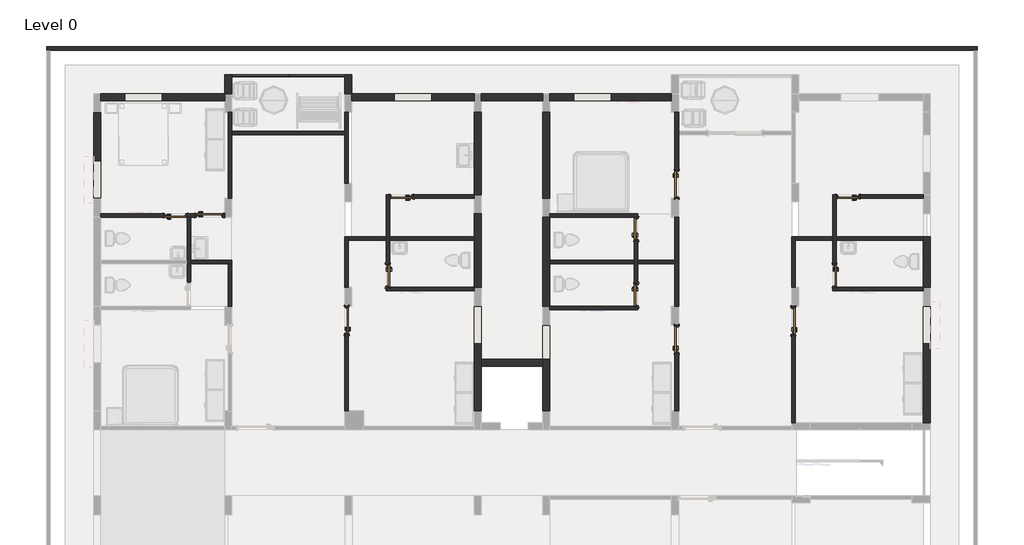
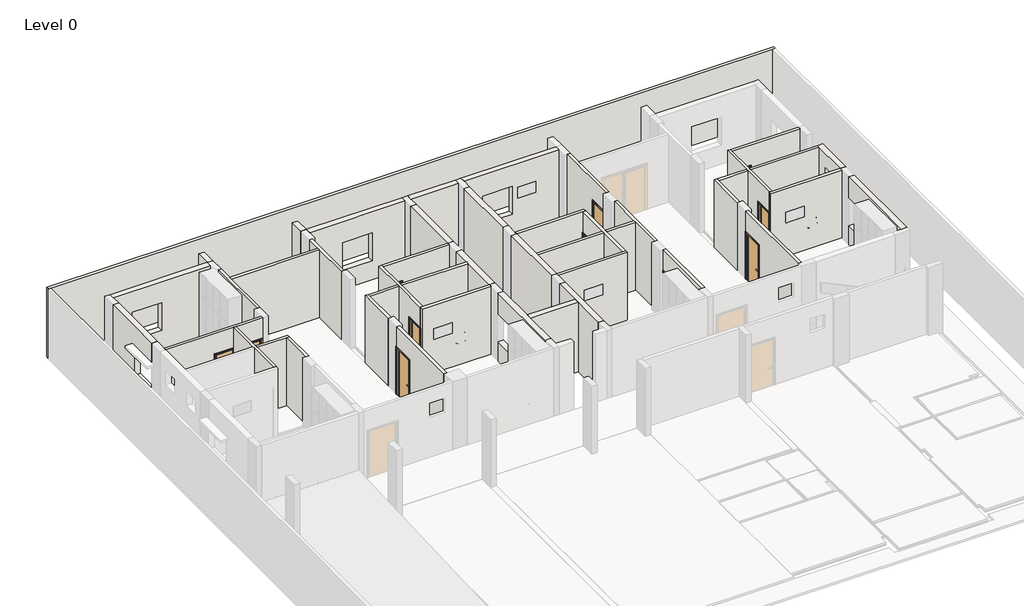
# One storey, part 2 of 6: 46 walls, 12 doors, 5 members, 2 plates.
"""IFC4 building model written with IfcOpenShell, lengths in millimetres."""

from ifc_helpers import new_model, si_unit, frame, origin, origin_with_axes, place, context, project, spatial, polyline, outline, extrude, faceted_brep, transform, mapped, element, save
from components import door_d225582b, door_4bb05ab8, doors_intsgl_3_11801b65, doors_intsgl_3_f3216364, rectangular_mullion_30mm_square_b78902bc, rectangular_mullion_30mm_square_5c6859bd, rectangular_mullion_30mm_square_457ab78e, rectangular_mullion_30mm_square_508dbaa4, system_panel_glazed_442d96c1, system_panel_glazed_6149afab

model = new_model("IFC4")

# Units and contexts
model_context = context("Model", 3, world=origin())
ifc_project = project(units=[si_unit("LENGTHUNIT", "METRE", prefix="MILLI")], contexts=[model_context])

# Site, building, storey
site = spatial("IfcSite", under=ifc_project)
building = spatial("IfcBuilding", under=site)
storey = spatial("IfcBuildingStorey", under=building, Name="Level 0", Elevation=0.0)

# Doors
placement = place(None, origin())
door_shape = door_d225582b(model_context)
element("IfcDoor", 1, ObjectType="Doors_IntSgl : 2'6\"", at=placement, inside=storey, context=model_context, shape_type="MappedRepresentation", body=[
    mapped(door_shape, transform((-10829.9825268, 6419.6522446, 0.0), x_axis=(1.0, 0.0, 0.0), y_axis=(0.0, 1.0, 0.0), z_axis=(0.0, 0.0, 1.0))),
])
element("IfcDoor", 2, ObjectType="Doors_IntSgl : 2'6\"", at=placement, inside=storey, context=model_context, shape_type="MappedRepresentation", body=[
    mapped(door_shape, transform((4085.7098461, 3836.3482139, 0.0), x_axis=(0.0, -1.0, 0.0), y_axis=(1.0, 0.0, 0.0), z_axis=(0.0, 0.0, 1.0))),
])
door_2_shape = door_4bb05ab8(model_context)
element("IfcDoor", 3, ObjectType="Doors_IntSgl : 2'6\"", at=placement, inside=storey, context=model_context, shape_type="MappedRepresentation", body=[
    mapped(door_2_shape, transform((-3954.0467595, 4470.172794, 0.0), x_axis=(-0.0005222285163052799, -0.9999998636386792, 0.0), y_axis=(0.9999998636386792, -0.0005222285163052799, 0.0), z_axis=(0.0, 0.0, 1.0))),
])
element("IfcDoor", 4, ObjectType="Doors_IntSgl : 2'6\"", at=placement, inside=storey, context=model_context, shape_type="MappedRepresentation", body=[
    mapped(door_2_shape, transform((-3514.5601716, 7029.4508507, 0.0), x_axis=(-0.9999998636386791, 0.000522228516302431, 0.0), y_axis=(-0.000522228516302431, -0.9999998636386791, 0.0), z_axis=(0.0, 0.0, 1.0))),
])
element("IfcDoor", 5, ObjectType="Doors_IntSgl : 2'6\"", at=placement, inside=storey, context=model_context, shape_type="MappedRepresentation", body=[
    mapped(door_2_shape, transform((4085.7098461, 5982.6482139, 0.0), x_axis=(0.0, 1.0, 0.0), y_axis=(-1.0, 0.0, 0.0), z_axis=(0.0, 0.0, 1.0))),
])
element("IfcDoor", 6, ObjectType="Doors_IntSgl : 2'6\"", at=placement, inside=storey, context=model_context, shape_type="MappedRepresentation", body=[
    mapped(door_2_shape, transform((10505.5598461, 4471.3482139, 0.0), x_axis=(0.0, -1.0, 0.0), y_axis=(1.0, 0.0, 0.0), z_axis=(0.0, 0.0, 1.0))),
])
element("IfcDoor", 7, ObjectType="Doors_IntSgl : 2'6\"", at=placement, inside=storey, context=model_context, shape_type="MappedRepresentation", body=[
    mapped(door_2_shape, transform((10943.7098461, 7030.3982139, 0.0), x_axis=(-1.0, 0.0, 0.0), y_axis=(0.0, -1.0, 0.0), z_axis=(0.0, 0.0, 1.0))),
])
doors_intsgl_3_shape = doors_intsgl_3_11801b65(model_context)
element("IfcDoor", 8, ObjectType="Doors_IntSgl : 3'", at=placement, inside=storey, context=model_context, shape_type="MappedRepresentation", body=[
    mapped(doors_intsgl_3_shape, transform((-9731.8901539, 6419.6522446, 0.0), x_axis=(1.0, 0.0, 0.0), y_axis=(0.0, 1.0, 0.0), z_axis=(0.0, 0.0, 1.0))),
])
element("IfcDoor", 9, ObjectType="Doors_IntSgl : 3'", at=placement, inside=storey, context=model_context, shape_type="MappedRepresentation", body=[
    mapped(doors_intsgl_3_shape, transform((5400.1598461, 2401.2482139, 0.0), x_axis=(0.0, 1.0, 0.0), y_axis=(-1.0, 0.0, 0.0), z_axis=(0.0, 0.0, 1.0))),
])
doors_intsgl_3_2_shape = doors_intsgl_3_f3216364(model_context)
element("IfcDoor", 10, ObjectType="Doors_IntSgl : 3'", at=placement, inside=storey, context=model_context, shape_type="MappedRepresentation", body=[
    mapped(doors_intsgl_3_2_shape, transform((-5287.3677108, 3023.5482139, 0.0), x_axis=(0.0, 1.0, 0.0), y_axis=(-1.0, 0.0, 0.0), z_axis=(0.0, 0.0, 1.0))),
])
element("IfcDoor", 11, ObjectType="Doors_IntSgl : 3'", at=placement, inside=storey, context=model_context, shape_type="MappedRepresentation", body=[
    mapped(doors_intsgl_3_2_shape, transform((5400.1598461, 7429.3022446, 0.0), x_axis=(0.0, -1.0, 0.0), y_axis=(1.0, 0.0, 0.0), z_axis=(0.0, 0.0, 1.0))),
])
element("IfcDoor", 12, ObjectType="Doors_IntSgl : 3'", at=placement, inside=storey, context=model_context, shape_type="MappedRepresentation", body=[
    mapped(doors_intsgl_3_2_shape, transform((9172.0598461, 2998.1482139, 0.0), x_axis=(0.0, 1.0, 0.0), y_axis=(-1.0, 0.0, 0.0), z_axis=(0.0, 0.0, 1.0))),
])

# Members
rectangular_mullion_30mm_square_shape = rectangular_mullion_30mm_square_b78902bc(model_context)
element("IfcMember", 13, ObjectType="Rectangular Mullion : 30mm_Square", at=placement, inside=storey, context=model_context, shape_type="MappedRepresentation", body=[
    mapped(rectangular_mullion_30mm_square_shape, transform((-7186.0406197, 10921.8022446, 1219.2), x_axis=(0.0, 0.0, 1.0), y_axis=(0.0, -1.0, 0.0), z_axis=(1.0, 0.0, 0.0))),
])
rectangular_mullion_30mm_square_2_shape = rectangular_mullion_30mm_square_5c6859bd(model_context)
element("IfcMember", 14, ObjectType="Rectangular Mullion : 30mm_Square", at=placement, inside=storey, context=model_context, shape_type="MappedRepresentation", body=[
    mapped(rectangular_mullion_30mm_square_2_shape, transform((-5374.0534022, 10921.8022446, 1219.2), x_axis=(0.0, 0.0, 1.0), y_axis=(0.0, -1.0, 0.0), z_axis=(1.0, 0.0, 0.0))),
])
rectangular_mullion_30mm_square_3_shape = rectangular_mullion_30mm_square_457ab78e(model_context)
element("IfcMember", 15, ObjectType="Rectangular Mullion : 30mm_Square", at=placement, inside=storey, context=model_context, shape_type="MappedRepresentation", body=[
    mapped(rectangular_mullion_30mm_square_3_shape, transform((-7171.0406197, 10921.8022446, 152.0481452), x_axis=(1.0, 0.0, 0.0), y_axis=(0.0, -1.0, 0.0), z_axis=(0.0, 0.0, -1.0))),
])
rectangular_mullion_30mm_square_4_shape = rectangular_mullion_30mm_square_508dbaa4(model_context)
element("IfcMember", 16, ObjectType="Rectangular Mullion : 30mm_Square", at=placement, inside=storey, context=model_context, shape_type="MappedRepresentation", body=[
    mapped(rectangular_mullion_30mm_square_4_shape, transform((-9001.04062, 10921.8022446, 1219.2), x_axis=(-1.0, 0.0, 0.0), y_axis=(0.0, -1.0, 0.0), z_axis=(0.0, 0.0, 1.0))),
])
element("IfcMember", 17, ObjectType="Rectangular Mullion : 30mm_Square", at=placement, inside=storey, context=model_context, shape_type="MappedRepresentation", body=[
    mapped(rectangular_mullion_30mm_square_4_shape, transform((-5344.0534022, 10921.8022446, 152.0481452), x_axis=(1.0, 0.0, 0.0), y_axis=(0.0, -1.0, 0.0), z_axis=(0.0, 0.0, -1.0))),
])

# Plates
system_panel_glazed_shape = system_panel_glazed_442d96c1(model_context)
element("IfcPlate", 18, ObjectType="System Panel : Glazed", at=placement, inside=storey, context=model_context, shape_type="MappedRepresentation", body=[
    mapped(system_panel_glazed_shape, transform((-8086.0406199, 10921.8022446, 152.0481452), x_axis=(1.0, 0.0, 0.0), y_axis=(0.0, 1.0, 0.0), z_axis=(0.0, 0.0, 1.0))),
])
system_panel_glazed_2_shape = system_panel_glazed_6149afab(model_context)
element("IfcPlate", 19, ObjectType="System Panel : Glazed", at=placement, inside=storey, context=model_context, shape_type="MappedRepresentation", body=[
    mapped(system_panel_glazed_2_shape, transform((-6257.547011, 10921.8022446, 152.0481452), x_axis=(1.0, 0.0, 0.0), y_axis=(0.0, 1.0, 0.0), z_axis=(0.0, 0.0, 1.0))),
])

# Walls
element("IfcWall", 20, ObjectType="2\"", at=placement, inside=storey, context=model_context, shape_type="SweptSolid", body=[
    extrude(outline(polyline([(-9001.04062, 10972.6022446), (-5344.0534022, 10972.6022446), (-5344.0534022, 10921.8022446), (-9001.04062, 10921.8022446), (-9001.04062, 10972.6022446)])), origin_with_axes(), (0.0, 0.0, 1.0), 152.0481452),
])
element("IfcWall", 21, ObjectType="9\"", at=placement, inside=storey, context=model_context, shape_type="SweptSolid", body=[
    extrude(outline(polyline([(0.0, -9230.2401539), (3048.0, -9230.2401539), (3048.0, -13249.7901539), (0.0, -13249.7901539), (0.0, -9230.2401539)]), holes=[polyline([(2133.6, -11248.7188871), (914.4, -11248.7188871), (914.4, -12467.9188871), (2133.6, -12467.9188871), (2133.6, -11248.7188871)])]), frame((0.0, 10133.2562752, 0.0), z_axis=(0.0, 1.0, 0.0), x_axis=(0.0, 0.0, 1.0)), (0.0, 0.0, 1.0), 228.6),
])
element("IfcWall", 22, ObjectType="9\"", at=placement, inside=storey, context=model_context, shape_type="SweptSolid", body=[
    extrude(outline(polyline([(0.0, -1153.0401539), (3048.0, -1153.0401539), (3048.0, -5115.4534022), (0.0, -5115.4534022), (0.0, -1153.0401539)]), holes=[polyline([(2133.6, -3743.8401538), (2133.6, -2524.6401538), (914.4, -2524.6401538), (914.4, -3743.8401538), (2133.6, -3743.8401538)])]), frame((0.0, 10134.4022446, 0.0), z_axis=(0.0, 1.0, 0.0), x_axis=(0.0, 0.0, 1.0)), (0.0, 0.0, 1.0), 228.6),
])
element("IfcWall", 23, ObjectType="9\"", at=placement, inside=storey, context=model_context, shape_type="SweptSolid", body=[
    extrude(outline(polyline([(1056.7598461, 10134.4022446), (-924.4401539, 10134.4022446), (-924.4401539, 10363.0022446), (1056.7598461, 10363.0022446), (1056.7598461, 10134.4022446)])), origin_with_axes(), (0.0, 0.0, 1.0), 3048.0),
])
element("IfcWall", 24, ObjectType="9\"", at=placement, inside=storey, context=model_context, shape_type="SweptSolid", body=[
    extrude(outline(polyline([(0.0, 1285.3598461), (0.0, 5228.7098461), (3048.0, 5228.7098461), (3048.0, 1285.3598461), (0.0, 1285.3598461)]), holes=[polyline([(2133.6, 3286.4311129), (914.4, 3286.4311129), (914.4, 2067.2311129), (2133.6, 2067.2311129), (2133.6, 3286.4311129)])]), frame((0.0, 10134.4022446, 0.0), z_axis=(0.0, 1.0, 0.0), x_axis=(0.0, 0.0, 1.0)), (0.0, 0.0, 1.0), 228.6),
])
element("IfcWall", 25, ObjectType="9\"", at=placement, inside=storey, context=model_context, shape_type="SweptSolid", body=[
    extrude(outline(polyline([(4090.3482139, 0.0), (4090.3482139, 3048.0), (5728.6482139, 3048.0), (5728.6482139, 0.0), (4090.3482139, 0.0)]), holes=[polyline([(5157.1482139, 2438.4), (4547.5482139, 2438.4), (4547.5482139, 1828.8), (5157.1482139, 1828.8), (5157.1482139, 2438.4)])]), frame((13382.1098465, 0.0, 0.0), z_axis=(1.0, 0.0, 0.0), x_axis=(0.0, 1.0, 0.0)), (0.0, 0.0, 1.0), 228.6),
])
element("IfcWall", 26, ObjectType="9\"", at=placement, inside=storey, context=model_context, shape_type="SweptSolid", body=[
    extrude(outline(polyline([(-3771.9, 0.0), (0.0, 0.0), (0.0, -3048.0), (-3771.9, -3048.0), (-3771.9, -2133.6), (-2552.7, -2133.6), (-2552.7, -914.4), (-3771.9, -914.4), (-3771.9, 0.0)])), frame((13382.1098461, -291.1517861, 0.0), z_axis=(1.0, -9.266855296587119e-11, 0.0), x_axis=(-9.266855296587119e-11, -1.0, 0.0)), (0.0, 0.0, 1.0), 228.6),
])
element("IfcWall", 27, ObjectType="9\"", at=placement, inside=storey, context=model_context, shape_type="SweptSolid", body=[
    extrude(outline(polyline([(9752.2562752, 0.0), (6972.1022446, 0.0), (6972.1022446, 914.4), (8190.1562752, 914.4), (8190.1562752, 2133.6), (6972.1022446, 2133.6), (6972.1022446, 3048.0), (9752.2562752, 3048.0), (9752.2562752, 0.0)])), frame((-13478.3901539, 0.0, 0.0), z_axis=(1.0, 0.0, 0.0), x_axis=(0.0, 1.0, 0.0)), (0.0, 0.0, 1.0), 228.6),
])
element("IfcWall", 28, ObjectType="9\"", at=placement, inside=storey, context=model_context, shape_type="SweptSolid", body=[
    extrude(outline(polyline([(-924.4401539, 7087.5482139), (-1153.0401539, 7087.5482139), (-1153.0401539, 9753.4022446), (-924.4401539, 9753.4022446), (-924.4401539, 7087.5482139)])), origin_with_axes(), (0.0, 0.0, 1.0), 3048.0),
])
element("IfcWall", 29, ObjectType="9\"", at=placement, inside=storey, context=model_context, shape_type="SweptSolid", body=[
    extrude(outline(polyline([(1056.7598461, 6972.1022446), (1056.7598461, 9753.4022446), (1285.3598461, 9753.4022446), (1285.3598461, 6972.1022446), (1056.7598461, 6972.1022446)])), origin_with_axes(), (0.0, 0.0, 1.0), 3048.0),
])
element("IfcWall", 30, ObjectType="9\"", at=placement, inside=storey, context=model_context, shape_type="SweptSolid", body=[
    extrude(outline(polyline([(1056.7598461, 3481.8941832), (1056.7598461, 6362.5022446), (1285.3598461, 6362.5022446), (1285.3598461, 3481.8941832), (1056.7598461, 3481.8941832)])), origin_with_axes(), (0.0, 0.0, 1.0), 3048.0),
])
element("IfcWall", 31, ObjectType="9\"", at=placement, inside=storey, context=model_context, shape_type="SweptSolid", body=[
    extrude(outline(polyline([(-1153.0401539, 4089.2022446), (-1153.0401539, 6477.9482139), (-924.4401539, 6477.9482139), (-924.4401539, 4089.2022446), (-1153.0401539, 4089.2022446)])), origin_with_axes(), (0.0, 0.0, 1.0), 3048.0),
])
element("IfcWall", 32, ObjectType="9\"", at=placement, inside=storey, context=model_context, shape_type="Brep", body=[
    faceted_brep([(-924.4401539, 89.8482139, 0.0), (-924.4401539, 1537.6482139, 0.0), (-924.4401539, 1766.2482139, 0.0), (-924.4401539, 3479.6022446, 0.0), (-924.4401539, 3479.6022446, 914.4), (-924.4401539, 2260.4022446, 914.4), (-924.4401539, 2260.4022446, 2133.6), (-924.4401539, 3479.6022446, 2133.6), (-924.4401539, 3479.6022446, 3048.0), (-924.4401539, 1766.2482139, 3048.0), (-924.4401539, 1537.6482139, 3048.0), (-924.4401539, 89.8482139, 3048.0), (-1153.0401539, 3479.6022446, 0.0), (-1153.0401539, 89.8482139, 0.0), (-1153.0401539, 89.8482139, 3048.0), (-1153.0401539, 3479.6022446, 3048.0), (-1153.0401539, 3479.6022446, 2133.6), (-1153.0401539, 2260.4022446, 2133.6), (-1153.0401539, 2260.4022446, 914.4), (-1153.0401539, 3479.6022446, 914.4)], [[[0, 1, 2, 3, 4, 5, 6, 7, 8, 9, 10, 11]], [[12, 13, 14, 15, 16, 17, 18, 19]], [[3, 2, 1, 0, 13, 12]], [[3, 12, 19, 4]], [[15, 8, 7, 16]], [[11, 10, 9, 8, 15, 14]], [[0, 11, 14, 13]], [[18, 5, 4, 19]], [[5, 18, 17, 6]], [[6, 17, 16, 7]]]),
])
element("IfcWall", 33, ObjectType="9\"", at=placement, inside=storey, context=model_context, shape_type="Brep", body=[
    faceted_brep([(1056.7598461, 2872.2941832, 0.0), (1056.7598461, 1766.2482139, 0.0), (1056.7598461, 1537.6482139, 0.0), (1056.7598461, 89.8482139, 0.0), (1056.7598461, 89.8482139, 3048.0), (1056.7598461, 1537.6482139, 3048.0), (1056.7598461, 1766.2482139, 3048.0), (1056.7598461, 2872.2941832, 3048.0), (1056.7598461, 2872.2941832, 2133.6), (1056.7598461, 1766.2482138, 2133.6), (1056.7598461, 1766.2482138, 914.4), (1056.7598461, 2872.2941832, 914.4), (1285.3598461, 89.8482139, 0.0), (1285.3598461, 2872.2941832, 0.0), (1285.3598461, 2872.2941832, 914.4), (1285.3598461, 1766.2482138, 914.4), (1285.3598461, 1766.2482138, 2133.6), (1285.3598461, 2872.2941832, 2133.6), (1285.3598461, 2872.2941832, 3048.0), (1285.3598461, 89.8482139, 3048.0)], [[[0, 1, 2, 3, 4, 5, 6, 7, 8, 9, 10, 11]], [[12, 13, 14, 15, 16, 17, 18, 19]], [[3, 2, 1, 0, 13, 12]], [[4, 3, 12, 19]], [[7, 6, 5, 4, 19, 18]], [[13, 0, 11, 14]], [[7, 18, 17, 8]], [[9, 16, 15, 10]], [[10, 15, 14, 11]], [[16, 9, 8, 17]]]),
])
element("IfcWall", 34, ObjectType="9\"", at=placement, inside=storey, context=model_context, shape_type="Brep", body=[
    faceted_brep([(-924.4401539, 1537.6482139, 0.0), (1056.7598461, 1537.6482139, 0.0), (1056.7598461, 1537.6482139, 3048.0), (-924.4401539, 1537.6482139, 3048.0), (-924.4401539, 1766.2482139, 0.0), (-924.4401539, 1766.2482139, 3048.0), (1056.7598461, 1766.2482139, 3048.0), (1056.7598461, 1766.2482139, 2133.6), (1056.7598461, 1766.2482139, 914.4), (1056.7598461, 1766.2482139, 0.0)], [[[0, 1, 2, 3]], [[4, 5, 6, 7, 8, 9]], [[1, 0, 4, 9]], [[2, 1, 9, 8, 7, 6]], [[3, 2, 6, 5]], [[0, 3, 5, 4]]]),
])
element("IfcWall", 35, ObjectType="9\"", at=placement, inside=storey, context=model_context, shape_type="Brep", body=[
    faceted_brep([(-9001.04062, 10361.8562752, 0.0), (-9001.04062, 10921.8022446, 0.0), (-9001.04062, 10972.6022446, 0.0), (-9001.04062, 10972.6022446, 152.0481452), (-9001.04062, 10972.6022446, 3048.0), (-9001.04062, 10361.8562752, 3048.0), (-9229.64062, 10361.8562752, 0.0), (-9229.64062, 10361.8562752, 3048.0), (-9229.64062, 10972.6022446, 3048.0), (-9229.64062, 10972.6022446, 0.0), (-9001.6401539, 10361.8562752, 0.0), (-9001.6401539, 10361.8562752, 3048.0)], [[[0, 1, 2, 3, 4, 5]], [[6, 7, 8, 9]], [[2, 1, 0, 10, 6, 9]], [[4, 3, 2, 9, 8]], [[5, 4, 8, 7, 11]], [[0, 5, 11, 7, 6, 10]]]),
])
element("IfcWall", 36, ObjectType="9\"", at=placement, inside=storey, context=model_context, shape_type="Brep", body=[
    faceted_brep([(-5115.4534022, 10364.1482139, 0.0), (-5115.4534022, 10972.6022446, 0.0), (-5115.4534022, 10972.6022446, 3048.0), (-5115.4534022, 10364.1482139, 3048.0), (-5344.0534022, 10364.1482139, 0.0), (-5344.0534022, 10364.1482139, 3048.0), (-5344.0534022, 10972.6022446, 3048.0), (-5344.0534022, 10972.6022446, 152.0481452), (-5344.0534022, 10972.6022446, 0.0), (-5344.0534022, 10921.8022446, 0.0)], [[[0, 1, 2, 3]], [[4, 5, 6, 7, 8, 9]], [[1, 0, 4, 9, 8]], [[2, 1, 8, 7, 6]], [[3, 2, 6, 5]], [[0, 3, 5, 4]]]),
])
element("IfcWall", 37, ObjectType="Brick Wall 4.5\"", at=placement, inside=storey, context=model_context, shape_type="SweptSolid", body=[
    extrude(outline(polyline([(0.0, -9230.2401539), (3048.0, -9230.2401539), (3048.0, -13249.7901539), (0.0, -13249.7901539), (0.0, -11210.9825268), (2133.6, -11210.9825268), (2133.6, -10448.9825268), (0.0, -10448.9825268), (0.0, -10189.0901539), (2133.6, -10189.0901539), (2133.6, -9274.6901539), (0.0, -9274.6901539), (0.0, -9230.2401539)])), frame((0.0, 6362.5022446, 0.0), z_axis=(0.0, 1.0, 0.0), x_axis=(0.0, 0.0, 1.0)), (0.0, 0.0, 1.0), 114.3),
])
element("IfcWall", 38, ObjectType="Brick Wall 4.5\"", at=placement, inside=storey, context=model_context, shape_type="SweptSolid", body=[
    extrude(outline(polyline([(6362.5617448, 3048.0), (6362.5617448, 0.0), (4241.6022446, 0.0), (4241.6022446, 2133.6), (3479.6022446, 2133.6), (3479.6022446, 3048.0), (6362.5617448, 3048.0)])), frame((-10450.1697227, 0.0, 0.0), z_axis=(1.0, 0.0, 0.0), x_axis=(0.0, 1.0, 0.0)), (0.0, 0.0, 1.0), 114.3),
])
element("IfcWall", 39, ObjectType="Brick Wall 4.5\"", at=placement, inside=storey, context=model_context, shape_type="Brep", body=[
    faceted_brep([(-10335.1401539, 4851.2022446, 0.0), (-9115.77783, 4851.2022446, 0.0), (-9001.47783, 4851.2022446, 0.0), (-9001.47783, 4851.2022446, 3048.0), (-9115.77783, 4851.2022446, 3048.0), (-10335.1401539, 4851.2022446, 3048.0), (-10335.1401539, 4965.5022446, 0.0), (-10335.1401539, 4965.5022446, 3048.0), (-9001.47783, 4965.5022446, 3048.0), (-9001.47783, 4965.5022446, 0.0)], [[[0, 1, 2, 3, 4, 5]], [[6, 7, 8, 9]], [[2, 1, 0, 6, 9]], [[3, 2, 9, 8]], [[5, 4, 3, 8, 7]], [[0, 5, 7, 6]]]),
])
element("IfcWall", 40, ObjectType="Brick Wall 4.5\"", at=placement, inside=storey, context=model_context, shape_type="SweptSolid", body=[
    extrude(outline(polyline([(89.8480892, 3048.0), (3480.7482139, 3048.0), (3480.7482139, 2133.6), (2566.3482139, 2133.6), (2566.3482139, 0.0), (89.8480892, 0.0), (89.8480892, 3048.0)])), frame((-5344.5177108, 0.0, 0.0), z_axis=(1.0, 0.0, 0.0), x_axis=(0.0, 1.0, 0.0)), (0.0, 0.0, 1.0), 114.3),
])
element("IfcWall", 41, ObjectType="Brick Wall 4.5\"", at=placement, inside=storey, context=model_context, shape_type="Brep", body=[
    faceted_brep([(-5229.7401539, 4089.2022446, 0.0), (-5229.7401539, 5613.2022446, 0.0), (-5229.7401539, 5727.5022446, 0.0), (-5229.7401539, 5727.5022446, 3048.0), (-5229.7401539, 5613.2022446, 3048.0), (-5229.7401539, 4089.2022446, 3048.0), (-5344.0401539, 4089.2022446, 0.0), (-5344.0401539, 4089.2022446, 3048.0), (-5344.0401539, 5727.5022446, 3048.0), (-5344.0401539, 5727.5022446, 0.0)], [[[0, 1, 2, 3, 4, 5]], [[6, 7, 8, 9]], [[2, 1, 0, 6, 9]], [[3, 2, 9, 8]], [[5, 4, 3, 8, 7]], [[0, 5, 7, 6]]]),
])
element("IfcWall", 42, ObjectType="Brick Wall 4.5\"", at=placement, inside=storey, context=model_context, shape_type="SweptSolid", body=[
    extrude(outline(polyline([(-4010.5401539, 5613.2022446), (-5229.7401539, 5613.2022446), (-5229.7401539, 5727.5022446), (-4010.5401539, 5727.5022446), (-4010.5401539, 5613.2022446)])), origin_with_axes(), (0.0, 0.0, 1.0), 3048.0),
])
element("IfcWall", 43, ObjectType="Brick Wall 4.5\"", at=placement, inside=storey, context=model_context, shape_type="Brep", body=[
    faceted_brep([(-4009.8304976, 7086.4020593, 3048.0), (-4009.8304976, 7086.4020593, 0.0), (-4010.5401539, 5727.5022446, 0.0), (-4010.5998446, 5613.2022446, 0.0), (-4010.9977826, 4851.2025875, 0.0), (-4010.9977826, 4851.2025875, 2133.6), (-4011.3957208, 4089.2026914, 2133.6), (-4011.3957208, 4089.2026914, 3048.0), (-4010.5998446, 5613.2022446, 3048.0), (-4010.5401539, 5727.5022446, 3048.0), (-3895.5305131, 7086.3423685, 0.0), (-3895.5305131, 7086.3423685, 3048.0), (-3896.2401383, 5727.5022446, 3048.0), (-3896.299829, 5613.2022446, 3048.0), (-3897.0957363, 4089.1430006, 3048.0), (-3897.0957363, 4089.1430006, 2133.6), (-3896.6977982, 4851.1428967, 2133.6), (-3896.6977982, 4851.1428967, 0.0), (-3896.299829, 5613.2022446, 0.0), (-3896.2401383, 5727.5022446, 0.0)], [[[0, 1, 2, 3, 4, 5, 6, 7, 8, 9]], [[10, 11, 12, 13, 14, 15, 16, 17, 18, 19]], [[1, 10, 19, 18, 17, 4, 3, 2]], [[14, 7, 6, 15]], [[7, 14, 13, 12, 11, 0, 9, 8]], [[1, 0, 11, 10]], [[5, 16, 15, 6]], [[16, 5, 4, 17]]]),
])
element("IfcWall", 44, ObjectType="Brick Wall 4.5\"", at=placement, inside=storey, context=model_context, shape_type="SweptSolid", body=[
    extrude(outline(polyline([(-1153.0401539, 5613.2022446), (-3896.2401539, 5613.2022446), (-3896.2401539, 5727.5022446), (-1153.0401539, 5727.5022446), (-1153.0401539, 5613.2022446)])), origin_with_axes(), (0.0, 0.0, 1.0), 3048.0),
])
element("IfcWall", 45, ObjectType="Brick Wall 4.5\"", at=placement, inside=storey, context=model_context, shape_type="SweptSolid", body=[
    extrude(outline(polyline([(1981.2001039, 0.0), (1981.2001039, -3048.0), (-761.2901203, -3048.0), (-761.2901203, -2133.6), (0.7098797, -2133.6), (0.7098797, 0.0), (1981.2001039, 0.0)])), frame((-3134.2999485, 6972.1022601, 0.0), z_axis=(0.0005222285163024312, 0.9999998636386791, 0.0), x_axis=(0.9999998636386791, -0.0005222285163024312, 0.0)), (0.0, 0.0, 1.0), 114.3),
])
element("IfcWall", 46, ObjectType="Brick Wall 4.5\"", at=placement, inside=storey, context=model_context, shape_type="Brep", body=[
    faceted_brep([(-9115.9401539, 9753.4022446, 0.0), (-9115.9401539, 6970.9562752, 0.0), (-9115.9401539, 6970.9562752, 3048.0), (-9115.9401539, 9753.4022446, 3048.0), (-9001.6401539, 9753.4022446, 0.0), (-9001.6401539, 9753.4022446, 3048.0), (-9001.6401539, 9143.8022446, 3048.0), (-9001.6401539, 9029.5022446, 3048.0), (-9001.6401539, 6970.9562752, 3048.0), (-9001.6401539, 6970.9562752, 0.0), (-9001.6401539, 9029.5022446, 0.0), (-9001.6401539, 9143.8022446, 0.0)], [[[0, 1, 2, 3]], [[4, 5, 6, 7, 8, 9, 10, 11]], [[1, 0, 4, 11, 10, 9]], [[2, 1, 9, 8]], [[3, 2, 8, 7, 6, 5]], [[0, 3, 5, 4]]]),
])
element("IfcWall", 47, ObjectType="Brick Wall 4.5\"", at=placement, inside=storey, context=model_context, shape_type="SweptSolid", body=[
    extrude(outline(polyline([(-5344.0401539, 9029.5022446), (-9001.6401539, 9029.5022446), (-9001.6401539, 9143.8022446), (-5344.0401539, 9143.8022446), (-5344.0401539, 9029.5022446)])), origin_with_axes(), (0.0, 0.0, 1.0), 3048.0),
])
element("IfcWall", 48, ObjectType="Brick Wall 4.5\"", at=placement, inside=storey, context=model_context, shape_type="Brep", body=[
    faceted_brep([(-5344.0401539, 9753.4022446, 0.0), (-5344.0401539, 9143.8022446, 0.0), (-5344.0401539, 9029.5022446, 0.0), (-5344.0401539, 7467.4022446, 0.0), (-5344.0401539, 7467.4022446, 3048.0), (-5344.0401539, 9029.5022446, 3048.0), (-5344.0401539, 9143.8022446, 3048.0), (-5344.0401539, 9753.4022446, 3048.0), (-5229.7401539, 9753.4022446, 0.0), (-5229.7401539, 9753.4022446, 3048.0), (-5229.7401539, 7467.4022446, 3048.0), (-5229.7401539, 7467.4022446, 0.0)], [[[0, 1, 2, 3, 4, 5, 6, 7]], [[8, 9, 10, 11]], [[3, 2, 1, 0, 8, 11]], [[4, 3, 11, 10]], [[7, 6, 5, 4, 10, 9]], [[0, 7, 9, 8]]]),
])
element("IfcWall", 49, ObjectType="Brick Wall 4.5\"", at=placement, inside=storey, context=model_context, shape_type="SweptSolid", body=[
    extrude(outline(polyline([(-1153.0401539, 3974.9022446), (-4010.5401539, 3974.9022446), (-4010.5401539, 4089.2022446), (-1153.0401539, 4089.2022446), (-1153.0401539, 3974.9022446)])), origin_with_axes(), (0.0, 0.0, 1.0), 3048.0),
])
element("IfcWall", 50, ObjectType="Brick Wall 4.5\"", at=placement, inside=storey, context=model_context, shape_type="SweptSolid", body=[
    extrude(outline(polyline([(-9115.77783, 3480.7482139), (-9115.77783, 4851.2022446), (-9001.47783, 4851.2022446), (-9001.47783, 3480.7482139), (-9115.77783, 3480.7482139)])), origin_with_axes(), (0.0, 0.0, 1.0), 3048.0),
])
element("IfcWall", 51, ObjectType="Brick Wall 4.5\"", at=placement, inside=storey, context=model_context, shape_type="Brep", body=[
    faceted_brep([(1285.3598461, 6363.6482139, 0.0), (4142.8598461, 6363.6482139, 0.0), (4142.8598461, 6363.6482139, 2133.6), (4142.8598461, 6363.6482139, 3048.0), (4028.5598461, 6363.6482139, 3048.0), (1285.3598461, 6363.6482139, 3048.0), (1285.3598461, 6477.9482139, 0.0), (1285.3598461, 6477.9482139, 3048.0), (4142.8598461, 6477.9482139, 3048.0), (4142.8598461, 6477.9482139, 0.0)], [[[0, 1, 2, 3, 4, 5]], [[6, 7, 8, 9]], [[1, 0, 6, 9]], [[3, 2, 1, 9, 8]], [[5, 4, 3, 8, 7]], [[0, 5, 7, 6]]]),
])
element("IfcWall", 52, ObjectType="Brick Wall 4.5\"", at=placement, inside=storey, context=model_context, shape_type="SweptSolid", body=[
    extrude(outline(polyline([(4028.5598461, 4852.3482139), (1285.3598461, 4852.3482139), (1285.3598461, 4966.6482139), (4028.5598461, 4966.6482139), (4028.5598461, 4852.3482139)])), origin_with_axes(), (0.0, 0.0, 1.0), 3048.0),
])
element("IfcWall", 53, ObjectType="Brick Wall 4.5\"", at=placement, inside=storey, context=model_context, shape_type="Brep", body=[
    faceted_brep([(1285.3598461, 3480.7482139, 0.0), (1285.3598461, 3480.7482139, 3048.0), (4028.5598461, 3480.7482139, 3048.0), (4142.8598461, 3480.7482139, 3048.0), (4142.8598461, 3480.7482139, 2133.6), (4028.5598461, 3480.7482139, 2133.6), (4028.5598461, 3480.7482139, 0.0), (1285.3598461, 3366.4482139, 0.0), (4142.8598461, 3366.4482139, 0.0), (4142.8598461, 3366.4482139, 3048.0), (1285.3598461, 3366.4482139, 3048.0), (4028.5598461, 3455.3482139, 0.0), (4142.8598461, 3455.3482139, 0.0), (4142.8598461, 3455.3482139, 2133.6), (4028.5598461, 3455.3482139, 2133.6)], [[[0, 1, 2, 3, 4, 5, 6]], [[7, 8, 9, 10]], [[8, 7, 0, 6, 11, 12]], [[1, 0, 7, 10]], [[3, 2, 1, 10, 9]], [[9, 8, 12, 13, 4, 3]], [[14, 11, 6, 5]], [[11, 14, 13, 12]], [[13, 14, 5, 4]]]),
])
element("IfcWall", 54, ObjectType="Brick Wall 4.5\"", at=placement, inside=storey, context=model_context, shape_type="Brep", body=[
    faceted_brep([(4028.5598461, 3480.7482139, 3048.0), (4028.5598461, 4852.3482139, 3048.0), (4028.5598461, 4966.6482139, 3048.0), (4028.5598461, 6363.6482139, 3048.0), (4028.5598461, 6363.6482139, 2133.6), (4028.5598461, 5601.6482139, 2133.6), (4028.5598461, 5601.6482139, 0.0), (4028.5598461, 4966.6482139, 0.0), (4028.5598461, 4852.3482139, 0.0), (4028.5598461, 4217.3482139, 0.0), (4028.5598461, 4217.3482139, 2133.6), (4028.5598461, 3480.7482139, 2133.6), (4142.8598461, 6363.6482139, 3048.0), (4142.8598461, 4966.6482139, 3048.0), (4142.8598461, 4852.3482139, 3048.0), (4142.8598461, 3480.7482139, 3048.0), (4142.8598461, 3480.7482139, 2133.6), (4142.8598461, 4217.3482139, 2133.6), (4142.8598461, 4217.3482139, 0.0), (4142.8598461, 4852.3482139, 0.0), (4142.8598461, 4966.6482139, 0.0), (4142.8598461, 5601.6482139, 0.0), (4142.8598461, 5601.6482139, 2133.6), (4142.8598461, 6363.6482139, 2133.6)], [[[0, 1, 2, 3, 4, 5, 6, 7, 8, 9, 10, 11]], [[12, 13, 14, 15, 16, 17, 18, 19, 20, 21, 22, 23]], [[6, 21, 20, 19, 18, 9, 8, 7]], [[15, 0, 11, 16]], [[3, 2, 1, 0, 15, 14, 13, 12]], [[3, 12, 23, 4]], [[22, 5, 4, 23]], [[5, 22, 21, 6]], [[10, 17, 16, 11]], [[17, 10, 9, 18]]]),
])
element("IfcWall", 55, ObjectType="Brick Wall 4.5\"", at=placement, inside=storey, context=model_context, shape_type="SweptSolid", body=[
    extrude(outline(polyline([(4142.8598461, 4966.6482139), (5343.0098461, 4966.6482139), (5343.0098461, 4852.3482139), (4142.8598461, 4852.3482139), (4142.8598461, 4966.6482139)])), origin_with_axes(), (0.0, 0.0, 1.0), 3048.0),
])
element("IfcWall", 56, ObjectType="Brick Wall 4.5\"", at=placement, inside=storey, context=model_context, shape_type="Brep", body=[
    faceted_brep([(5457.3098461, 3480.7482139, 0.0), (5457.3098461, 6362.5022446, 0.0), (5457.3098461, 6362.5022446, 3048.0), (5457.3098461, 3480.7482139, 3048.0), (5343.0098461, 3480.7482139, 0.0), (5343.0098461, 3480.7482139, 3048.0), (5343.0098461, 4852.3482139, 3048.0), (5343.0098461, 4966.6482139, 3048.0), (5343.0098461, 6362.5022446, 3048.0), (5343.0098461, 6362.5022446, 0.0), (5343.0098461, 4966.6482139, 0.0), (5343.0098461, 4852.3482139, 0.0)], [[[0, 1, 2, 3]], [[4, 5, 6, 7, 8, 9, 10, 11]], [[1, 0, 4, 11, 10, 9]], [[2, 1, 9, 8]], [[3, 2, 8, 7, 6, 5]], [[0, 3, 5, 4]]]),
])
element("IfcWall", 57, ObjectType="Brick Wall 4.5\"", at=placement, inside=storey, context=model_context, shape_type="SweptSolid", body=[
    extrude(outline(polyline([(6972.1022446, 3048.0), (9753.4022446, 3048.0), (9753.4022446, 0.0), (7886.5022446, 0.0), (7886.5022446, 2133.6), (6972.1022446, 2133.6), (6972.1022446, 3048.0)])), frame((5343.0098461, 0.0, 0.0), z_axis=(1.0, 0.0, 0.0), x_axis=(0.0, 1.0, 0.0)), (0.0, 0.0, 1.0), 114.3),
])
element("IfcWall", 58, ObjectType="Brick Wall 4.5\"", at=placement, inside=storey, context=model_context, shape_type="SweptSolid", body=[
    extrude(outline(polyline([(0.0, 13382.1098461), (3048.0, 13382.1098461), (3048.0, 10562.7098461), (2133.6, 10562.7098461), (2133.6, 11324.7098461), (0.0, 11324.7098461), (0.0, 13382.1098461)])), frame((0.0, 6973.2482139, 0.0), z_axis=(0.0, 1.0, 0.0), x_axis=(0.0, 0.0, 1.0)), (0.0, 0.0, 1.0), 114.3),
])
element("IfcWall", 59, ObjectType="Brick Wall 4.5\"", at=placement, inside=storey, context=model_context, shape_type="Brep", body=[
    faceted_brep([(10562.7098461, 7087.5482139, 0.0), (10562.7098461, 7087.5482139, 3048.0), (10562.7098461, 5728.6482139, 3048.0), (10562.7098461, 5614.3482139, 3048.0), (10562.7098461, 4090.3482139, 3048.0), (10562.7098461, 4090.3482139, 2133.6), (10562.7098461, 4852.3482139, 2133.6), (10562.7098461, 4852.3482139, 0.0), (10562.7098461, 5614.3482139, 0.0), (10562.7098461, 5728.6482139, 0.0), (10448.4098461, 7087.5482139, 3048.0), (10448.4098461, 7087.5482139, 0.0), (10448.4098461, 5728.6482139, 0.0), (10448.4098461, 5614.3482139, 0.0), (10448.4098461, 4852.3482139, 0.0), (10448.4098461, 4852.3482139, 2133.6), (10448.4098461, 4090.3482139, 2133.6), (10448.4098461, 4090.3482139, 3048.0), (10448.4098461, 5614.3482139, 3048.0), (10448.4098461, 5728.6482139, 3048.0), (10448.8158558, 4090.3482139, 3048.0)], [[[0, 1, 2, 3, 4, 5, 6, 7, 8, 9]], [[10, 11, 12, 13, 14, 15, 16, 17, 18, 19]], [[11, 0, 9, 8, 7, 14, 13, 12]], [[1, 0, 11, 10]], [[4, 3, 2, 1, 10, 19, 18, 17, 20]], [[4, 20, 17, 16, 5]], [[15, 6, 5, 16]], [[6, 15, 14, 7]]]),
])
element("IfcWall", 60, ObjectType="Brick Wall 4.5\"", at=placement, inside=storey, context=model_context, shape_type="SweptSolid", body=[
    extrude(outline(polyline([(13382.1098465, 5728.6482139), (13382.1098465, 5614.3482139), (10562.7098461, 5614.3482139), (10562.7098461, 5728.6482139), (13382.1098465, 5728.6482139)])), origin_with_axes(), (0.0, 0.0, 1.0), 3048.0),
    extrude(outline(polyline([(9229.2098461, 5614.3482139), (9229.2098461, 5728.6482139), (10448.4098461, 5728.6482139), (10448.4098461, 5614.3482139), (9229.2098461, 5614.3482139)])), origin_with_axes(), (0.0, 0.0, 1.0), 3048.0),
])
element("IfcWall", 61, ObjectType="Brick Wall 4.5\"", at=placement, inside=storey, context=model_context, shape_type="Brep", body=[
    faceted_brep([(9114.9098461, 5728.6482139, 0.0), (9114.9098461, 4090.3482139, 0.0), (9114.9098461, 4090.3482139, 3048.0), (9114.9098461, 5728.6482139, 3048.0), (9229.2098461, 5728.6482139, 0.0), (9229.2098461, 5728.6482139, 3048.0), (9229.2098461, 5614.3482139, 3048.0), (9229.2098461, 4090.3482139, 3048.0), (9229.2098461, 4090.3482139, 0.0), (9229.2098461, 5614.3482139, 0.0)], [[[0, 1, 2, 3]], [[4, 5, 6, 7, 8, 9]], [[1, 0, 4, 9, 8]], [[2, 1, 8, 7]], [[3, 2, 7, 6, 5]], [[0, 3, 5, 4]]]),
])
element("IfcWall", 62, ObjectType="Brick Wall 4.5\"", at=placement, inside=storey, context=model_context, shape_type="Brep", body=[
    faceted_brep([(10448.8158558, 3976.0482139, 0.0), (13382.1098461, 3976.0482139, 0.0), (13382.1098461, 3976.0482139, 3048.0), (10448.8158558, 3976.0482139, 3048.0), (10448.8158558, 4090.3482139, 0.0), (10448.8158558, 4090.3482139, 3048.0), (10562.7098461, 4090.3482139, 3048.0), (13382.1098461, 4090.3482139, 3048.0), (13382.1098461, 4090.3482139, 0.0)], [[[0, 1, 2, 3]], [[4, 5, 6, 7, 8]], [[1, 0, 4, 8]], [[2, 1, 8, 7]], [[3, 2, 7, 6, 5]], [[0, 3, 5, 4]]]),
])
element("IfcWall", 63, ObjectType="Brick Wall 4.5\"", at=placement, inside=storey, context=model_context, shape_type="SweptSolid", body=[
    extrude(outline(polyline([(-291.1517861, 0.0), (-291.1517861, 3048.0), (3480.7482139, 3048.0), (3480.7482139, 0.0), (3455.3482139, 0.0), (3455.3482139, 2133.6), (2540.9482139, 2133.6), (2540.9482139, 0.0), (-291.1517861, 0.0)])), frame((9114.9098461, 0.0, 0.0), z_axis=(1.0, 0.0, 0.0), x_axis=(0.0, 1.0, 0.0)), (0.0, 0.0, 1.0), 114.3),
])
element("IfcWall", 64, ObjectType="Brick Wall 4.5\"", at=placement, inside=storey, context=model_context, shape_type="SweptSolid", body=[
    extrude(outline(polyline([(2871.1482139, 3048.0), (2871.1482139, 0.0), (2858.4482139, 0.0), (2858.4482139, 2133.6), (1944.0482139, 2133.6), (1944.0482139, 0.0), (89.8482139, 0.0), (89.8482139, 3048.0), (2871.1482139, 3048.0)])), frame((5343.0098461, 0.0, 0.0), z_axis=(1.0, 0.0, 0.0), x_axis=(0.0, 1.0, 0.0)), (0.0, 0.0, 1.0), 114.3),
])
element("IfcWall", 65, ObjectType="Shear Wall 4.5\" 2", at=placement, inside=storey, context=model_context, shape_type="Brep", body=[
    faceted_brep([(15134.7098461, 11888.1482139, 0.0), (-15002.3901539, 11888.1482139, 0.0), (-15002.3901539, 11888.1482139, 3048.0), (15134.7098461, 11888.1482139, 3048.0), (15134.7098461, 11773.8482139, 0.0), (15134.7098461, 11773.8482139, 3048.0), (15020.4098461, 11773.8482139, 3048.0), (-14888.0901539, 11773.8482139, 3048.0), (-15002.3901539, 11773.8482139, 3048.0), (-15002.3901539, 11773.8482139, 0.0), (-14888.0901539, 11773.8482139, 0.0), (15020.4098461, 11773.8482139, 0.0)], [[[0, 1, 2, 3]], [[4, 5, 6, 7, 8, 9, 10, 11]], [[1, 0, 4, 11, 10, 9]], [[2, 1, 9, 8]], [[3, 2, 8, 7, 6, 5]], [[0, 3, 5, 4]]]),
])

save(model, "model.ifc")

# Revit data of these elements
# Type "Doors_IntSgl : 2'6\""
#   Type Mark = "48"
#   Type Comments = "Internal Single"
#   Operation = "SingleSwingRight"
#   Manufacturer = "Revit"
#   Keynote = "L20"
#   Description = "Internal Single Door"
#   Analytic Construction = "Metal"
#   UnderCut = 0' - 0.31496"
#   Tolerance = 0' - 0.07874"
#   Thickness = 0' - 1.49606"
#   Thermal Resistance (R) = 0.270117 (m²·K)/W
#   Structural Tolerance = 0' - 0.31496"
#   StopDepth = 0' - 1.25984"
#   Stop Thickness = 0' - 0.74803"
#   Rough Width = 2' - 6"
#   Rough Height = 7' - 0"
#   Height to Top Lock Rail = 3' - 3.37008"
#   Heat Transfer Coefficient (U) = 3.7021 W/(m²·K)
#   Handle Z Distance = 2' - 11.43307"
#   Handle X Distance = 0' - 2.95276"
#   Frame Thickness = 0' - 1.25984"
#   Door Panel Width = 2' - 2.69291"
#   Door Panel Thickness = 0' - 1.49606"
#   Door Panel Offset = 0' - 0"
#   Height = 7' - 0"
#   Width = 2' - 6"
#   Door Panel Height = 6' - 10.0315"
#   Architrave Setback = 0' - 0.19685"
#   Vis - Ironmongery = yes
#   Material Ironmongery = Door - Handle
#   Material Frame = Door - Frame/Mullion (1)
#   Material Door = Door - Panel
#   Material Architrave = Door - Architrave
#   Visual Light Transmittance = 0
#   Solar Heat Gain Coefficient = 0
#   Function = (empty or 0)
#   Wall Closure = (empty or 0)
# Type "Doors_IntSgl : 3'"
#   Type Mark = "47"
#   Type Comments = "Internal Single"
#   Operation = "SingleSwingRight"
#   Manufacturer = "Revit"
#   Keynote = "L20"
#   Description = "Internal Single Door"
#   Analytic Construction = "Metal"
#   UnderCut = 0' - 0.31496"
#   Tolerance = 0' - 0.07874"
#   Thickness = 0' - 1.49606"
#   Thermal Resistance (R) = 0.270117 (m²·K)/W
#   Structural Tolerance = 0' - 0.31496"
#   StopDepth = 0' - 1.25984"
#   Stop Thickness = 0' - 0.74803"
#   Rough Width = 3' - 0"
#   Rough Height = 7' - 0"
#   Height to Top Lock Rail = 3' - 3.37008"
#   Heat Transfer Coefficient (U) = 3.7021 W/(m²·K)
#   Handle Z Distance = 2' - 11.43307"
#   Handle X Distance = 0' - 2.95276"
#   Frame Thickness = 0' - 1.25984"
#   Door Panel Width = 2' - 8.69291"
#   Door Panel Thickness = 0' - 1.49606"
#   Door Panel Offset = 0' - 0"
#   Height = 7' - 0"
#   Width = 3' - 0"
#   Door Panel Height = 6' - 10.0315"
#   Architrave Setback = 0' - 0.19685"
#   Vis - Ironmongery = yes
#   Material Ironmongery = Door - Handle
#   Material Frame = Door - Frame/Mullion (1)
#   Material Door = Door - Panel
#   Material Architrave = Door - Architrave
#   Visual Light Transmittance = 0
#   Solar Heat Gain Coefficient = 0
#   Function = (empty or 0)
#   Wall Closure = (empty or 0)
# Type "Rectangular Mullion : 30mm_Square"
#   Keynote = "H11"
#   built-in parameter 1007304 = 0.0984252 (stored number, unit not read)
#   built-in parameter 1007301 = 0.0492126 (stored number, unit not read)
#   built-in parameter 1007300 = 0.0492126 (stored number, unit not read)
# Type "System Panel : Glazed"
#   Keynote = "H11"
#   Construction Type Id = "GSP4R"
#   Analytic Construction = "1/8 in Pilkington single glazing"
#   Visual Light Transmittance = 0.9
#   Solar Heat Gain Coefficient = 0.86
#   Heat Transfer Coefficient (U) = 6.7069 W/(m²·K)
#   Define Thermal Properties by = 1
# Type "2\""
#   Keynote = "F10"
#   Layers, outside or top first: 0' - 2" "Concrete" (function 1)
# Type "9\""
#   Keynote = "F10"
#   Layers, outside or top first: 0' - 9" "Concrete" (function 1)
# Type "Brick Wall 4.5\""
#   Keynote = "F10"
#   Layers, outside or top first: 0' - 4 1/2" "Brick, Engineering" (function 1)
# Type "Shear Wall 4.5\" 2"
#   Keynote = "F10"
#   Layers, outside or top first: 0' - 4 1/2" "Concrete Masonry Units _High Density" (function 1)
# Elements 1, 2, 3, 4, 5, 6, 7 (IfcDoor, "Doors_IntSgl : 2'6\"")
#   Phase Created = New Construction
#   Materials on its faces: "Door - Architrave", "Door - Handle", "Door - Frame/Mullion (1)", "Door - Panel"
# Elements 8, 9, 10, 11, 12 (IfcDoor, "Doors_IntSgl : 3'")
#   Phase Created = New Construction
#   Materials on its faces: "Door - Architrave", "Door - Handle", "Door - Frame/Mullion (1)", "Door - Panel"
# Elements 13, 14, 15, 16, 17 (IfcMember, "Rectangular Mullion : 30mm_Square")
#   Phase Created = New Construction
#   Materials on its faces: "Aluminium"
# Elements 18, 19 (IfcPlate, "System Panel : Glazed")
#   Phase Created = New Construction
#   Materials on its faces: "Glass"
# Element 20 (IfcWall, "2\"")
#   Top Offset = 0' - 0"
#   Base Offset = 0' - 0"
#   Unconnected Height = 0' - 5.98615"
#   wall height = 0' - 5.98615"
#   Phase Created = New Construction
#   Base Constraint = Level 0
#   Materials on its faces: "Concrete"
# Elements 21, 22, 23, 24, 25, 26, 27, 28, 29, 30, 31, 32, 33, 34, 35, 36 (IfcWall, "9\"")
#   Top Offset = 0' - 0"
#   Base Offset = 0' - 0"
#   wall height = 10' - 0"
#   Phase Created = New Construction
#   Base Constraint = Level 0
#   Top Constraint = Level 1
#   Materials on its faces: "Concrete"
# Elements 37, 38, 39, 40, 41, 42, 43, 44, 45, 46, 47, 48, 49, 50, 51, 52, 53, 54, 55, 56, 57, 58, 59, 60, 61, 62, 63, 64 (IfcWall, "Brick Wall 4.5\"")
#   Top Offset = 0' - 0"
#   Base Offset = 0' - 0"
#   wall height = 10' - 0"
#   Phase Created = New Construction
#   Base Constraint = Level 0
#   Top Constraint = Level 1
#   Materials on its faces: "Brick, Engineering"
# Element 65 (IfcWall, "Shear Wall 4.5\" 2")
#   Top Offset = 0' - 0"
#   Base Offset = 0' - 0"
#   wall height = 10' - 0"
#   Phase Created = New Construction
#   Base Constraint = Level 0
#   Top Constraint = Level 1
#   Materials on its faces: "Concrete Masonry Units _High Density"
# Materials
#   "Door - Handle": colour RGB 0 0 0, transparency 0, Keynote = "P21", Cost = 0
#   "Door - Frame/Mullion (1)": class "Wood", colour RGB 212 179 113, transparency 0, Keynote = "L20", Cost = 0
#   "Door - Panel": class "Wood", colour RGB 210 159 95, transparency 0, Keynote = "L20", Cost = 0
#   "Door - Architrave": class "Wood", colour RGB 154 90 5, transparency 0, Keynote = "P20", Cost = 0
#   "Concrete": class "Concrete", colour RGB 120 120 120, transparency 0, Description = "Portland Cement Concrete", Cost = 0
#   "Brick, Engineering": class "Masonry", colour RGB 255 125 125, transparency 0, Description = "High fired, dense brick", Cost = 0
#   "Concrete Masonry Units _High Density": class "Masonry", colour RGB 181 181 181, transparency 0, Description = "Concrete masonry units", Cost = 0
#   "Aluminium": class "Metal", colour RGB 247 247 247, transparency 0, Description = "Aluminium 6061", Cost = 0
#   "Glass": class "Glass", colour RGB 0 128 192, transparency 0.9, Description = "Soda Lime Glass", Cost = 0
